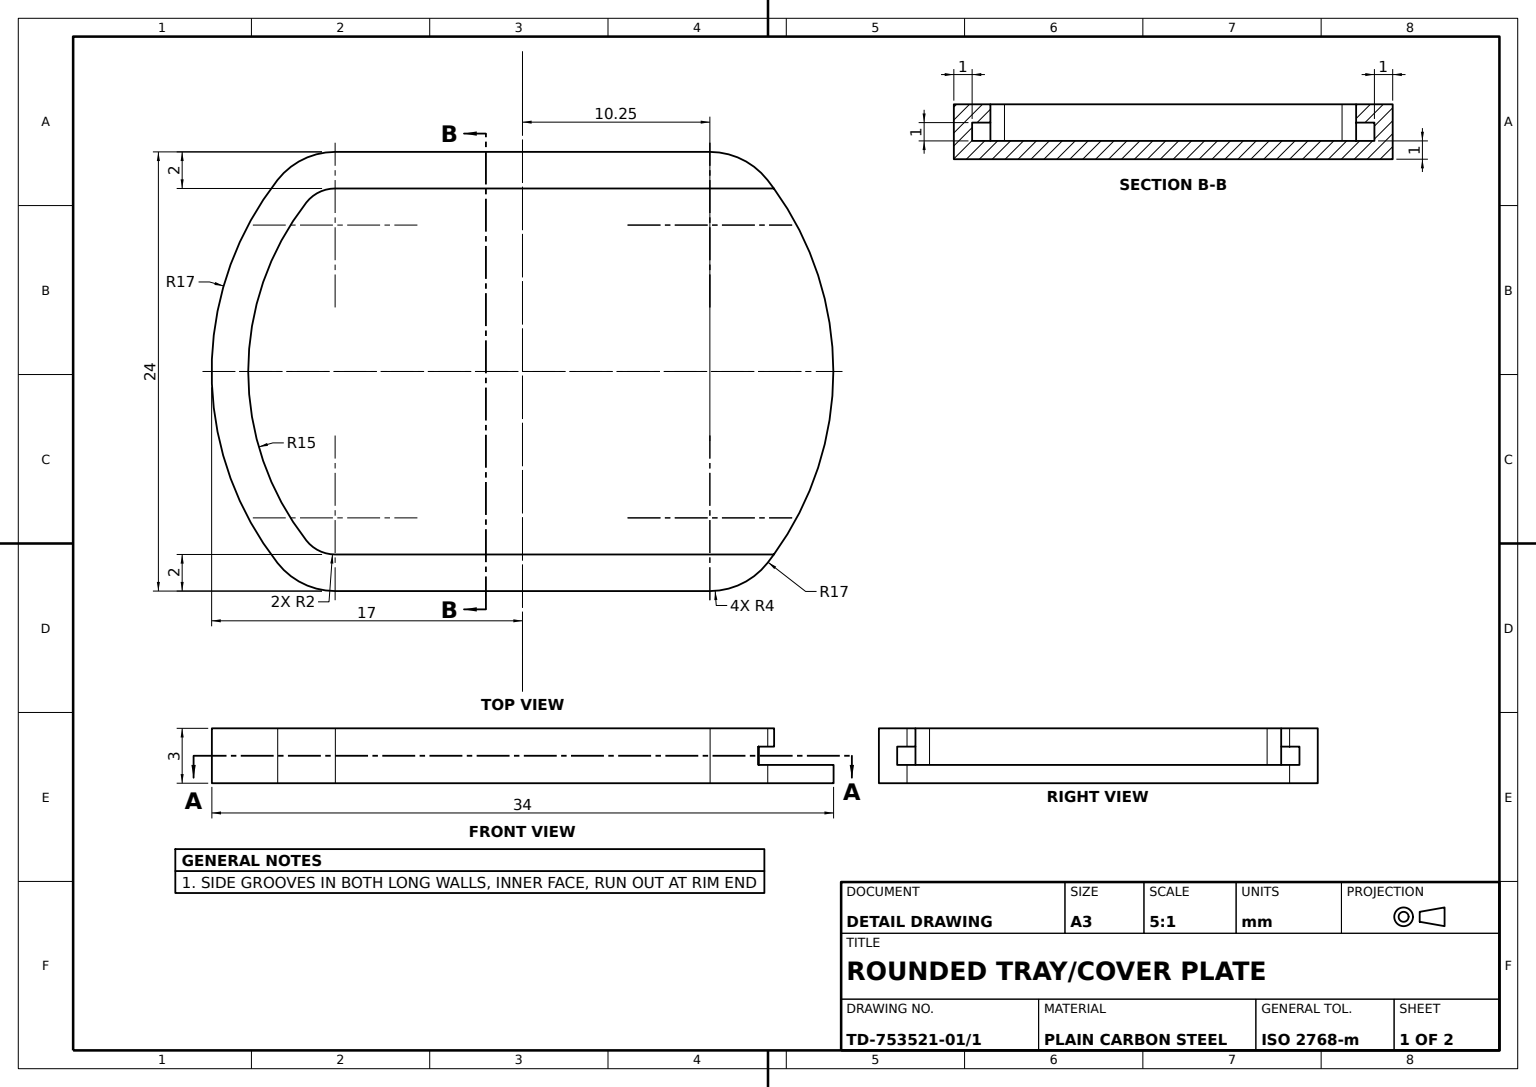
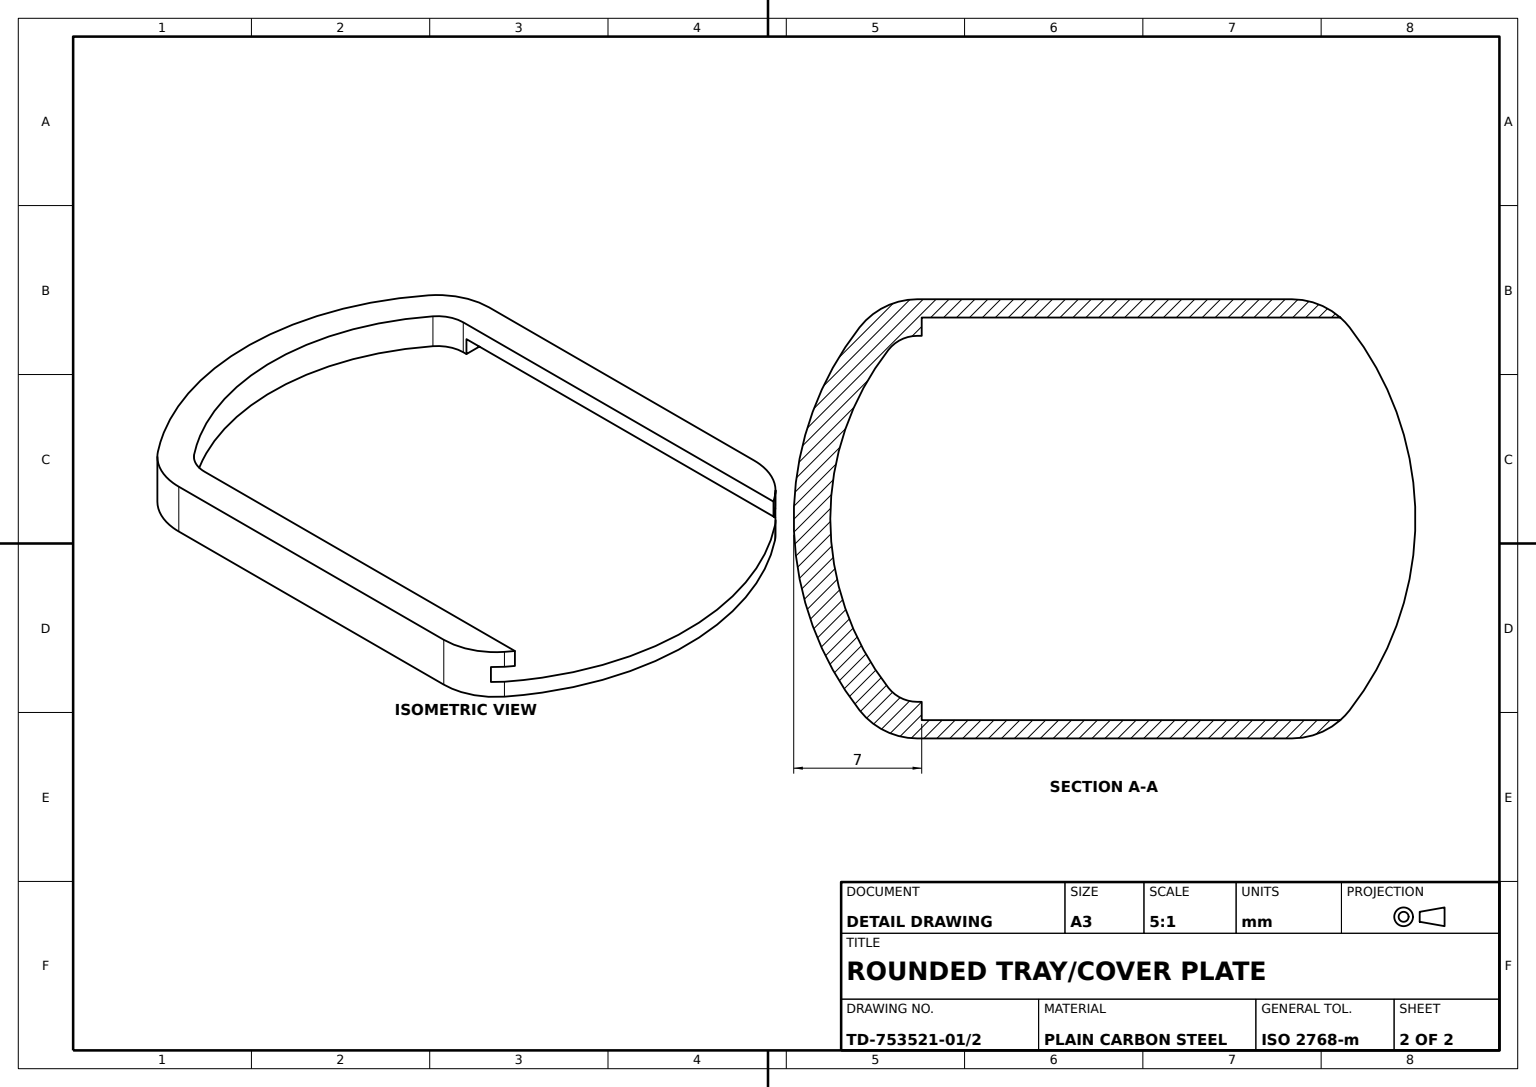
SolidWorks part; units mm, degrees
material "Plain Carbon Steel"
ref_plane "Front Plane" through (0, 0, 0) normal (0, 0, 1) x (1, 0, 0)
ref_plane "Top Plane" through (0, 0, 0) normal (0, 1, 0) x (1, 0, 0)
ref_plane "Right Plane" through (0, 0, 0) normal (1, 0, 0) x (0, 0, -1)
sketch "Base Plate Sketch" plane through (0, 0, 0) normal (0, 1, 0) x (1, 0, 0)
  line L0 (0, 0) -> (0, 7.2132)
  line L1 (-10.247, 12) -> (10.247, 12)
  line L2 (-10.247, -12) -> (10.247, -12)
  arc A0 (-13.3999, 10.4615) -> (-13.3999, -10.4615) centre (0, 0) ccw
  arc A1 (13.3999, -10.4615) -> (10.247, -12) centre (10.247, -8) cw
  arc A2 (-13.3999, -10.4615) -> (-10.247, -12) centre (-10.247, -8) ccw
  arc A3 (-13.3999, 10.4615) -> (-10.247, 12) centre (-10.247, 8) cw
  arc A4 (13.3999, 10.4615) -> (10.247, 12) centre (10.247, 8) ccw
  arc A5 (13.3999, 10.4615) -> (13.3999, -10.4615) centre (0, 0) cw
  dimension "D1" = 34
  dimension "D2" = 4
  dimension "D3" = 10.247
  dimension "D4" = 19.2132
extrude "Base Plate" add sketch "Base Plate Sketch" along normal blind 1
sketch "Rim Wall Sketch" plane through (0, 1, 0) normal (0, 1, 0) x (1, 0, 0)
  line L12 (-10.247, -10) -> (10.247, -10)
  line L13 (10.247, 10) -> (-10.247, 10)
  line L14 (-10.247, -10) -> (13.7477, -10)
  line L15 (13.7477, 10) -> (-10.247, 10)
  line L16 (-10.247, -12) -> (10.247, -12)
  line L17 (10.247, 12) -> (-10.247, 12)
  arc A23 (11.8234, 9.2308) -> (10.247, 10) centre (10.247, 8) ccw
  arc A24 (10.247, -10) -> (11.8234, -9.2308) centre (10.247, -8) ccw
  arc A25 (-11.8234, -9.2308) -> (-10.247, -10) centre (-10.247, -8) ccw
  arc A26 (-10.247, 10) -> (-11.8234, 9.2308) centre (-10.247, 8) ccw
  arc A27 (-11.8234, 9.2308) -> (-11.8234, -9.2308) centre (0, 0) ccw
  arc A29 (-10.247, 12) -> (-13.3999, 10.4615) centre (-10.247, 8) ccw
  arc A30 (-11.8234, -9.2308) -> (-10.247, -10) centre (-10.247, -8) ccw
  arc A31 (-10.247, 10) -> (-11.8234, 9.2308) centre (-10.247, 8) ccw
  arc A32 (-11.8234, 9.2308) -> (-11.8234, -9.2308) centre (0, 0) ccw
  arc A33 (-13.3999, 10.4615) -> (-13.3999, -10.4615) centre (0, 0) ccw
  arc A34 (-13.3999, -10.4615) -> (-10.247, -12) centre (-10.247, -8) ccw
  arc A35 (10.247, -12) -> (13.3999, -10.4615) centre (10.247, -8) ccw
  arc A36 (13.3999, -10.4615) -> (13.3999, 10.4615) centre (0, 0) ccw
  arc A37 (13.3999, 10.4615) -> (10.247, 12) centre (10.247, 8) ccw
  arc M16 (13.3999, -10.4615) -> (13.3999, 10.4615) centre (0, 0) ccw
  arc M17 (13.3999, 10.4615) -> (10.247, 12) centre (10.247, 8) ccw
  line M18 (10.247, 12) -> (-10.247, 12)
  arc M19 (-10.247, 12) -> (-13.3999, 10.4615) centre (-10.247, 8) ccw
  arc M20 (-13.3999, 10.4615) -> (-13.3999, -10.4615) centre (0, 0) ccw
  arc M21 (-13.3999, -10.4615) -> (-10.247, -12) centre (-10.247, -8) ccw
  line M22 (-10.247, -12) -> (10.247, -12)
  arc M23 (10.247, -12) -> (13.3999, -10.4615) centre (10.247, -8) ccw
  dimension "D1" = 2
extrude "Rim Wall" add sketch "Rim Wall Sketch" along normal blind 2 contours A32 A31 L15 L14 A30 M16 M17 M18 M19 M20 M21 M22 M23
ref_plane "Groove Section Plane" through (30, 0, 0) normal (1, 0, 0) x (0, 0, -1)
sketch "Side Groove A Sketch" plane through (30, 0, 0) normal (1, 0, 0) x (0, 0, -1)
  line L0 (-10, 3) -> (-10, 1) construction
  line L1 (-10, 2) -> (-11, 2)
  line L2 (-10, 2) -> (-10, 1)
  line L3 (-10, 1) -> (-11, 1)
  line L4 (-11, 2) -> (-11, 1)
  line L5 (-12, 3) -> (-12, 0) construction
  line L6 (-10, 3) -> (-10.4615, 3) construction
  dimension "D1" = 1
  dimension "D2" = 1
  dimension "D3" = 2
extrude "Side Groove A" cut sketch "Side Groove A Sketch" against normal blind 40
sketch "Side Groove B Sketch" plane through (30, 0, 0) normal (1, 0, 0) x (0, 0, -1)
  line L0 (12, 3) -> (12, 0) construction
  line L1 (10, 1) -> (11, 1)
  line L2 (10, 1) -> (10, 2)
  line L3 (10, 2) -> (11, 2)
  line L4 (11, 1) -> (11, 2)
  line L6 (12, 3) -> (10.4615, 3) construction
  dimension "D1" = 1
  dimension "D2" = 1
extrude "Side Groove B" cut sketch "Side Groove B Sketch" against normal blind 40
